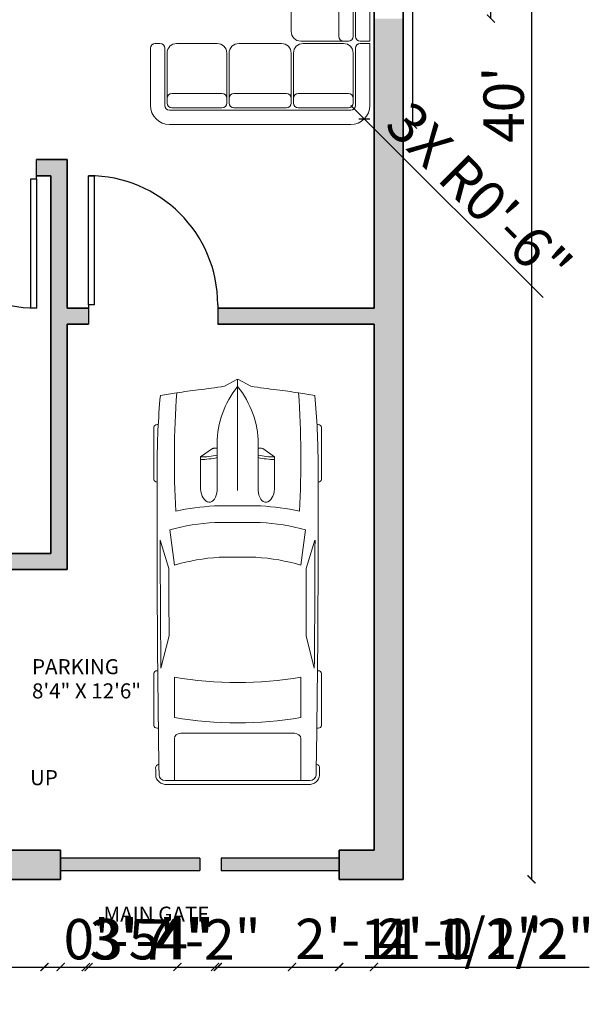
# Model space of a CAD drawing. Units: inches. Extents: x 1750 to 7466, y 1409 to 2004.
# Tile 2 of 5: x 1975 to 2152, y 1409 to 1715. Entities that reach past the tile are written whole.
import ezdxf

# ---------------------------------------------------------------- set-up
doc = ezdxf.new("R2010")
doc.units = ezdxf.units.IN
for name, color, linetype, lineweight in [('A-ANNO-DIMS', 2, 'Continuous', 18), ('A-ANNO-TEXT', 7, 'Continuous', 18), ('A-AREA-IDEN', 7, 'Continuous', 18), ('A-DOOR', 3, 'Continuous', 25), ('A-FURN', 8, 'Continuous', 18), ('A-SITE-PARK', 8, 'Continuous', 13), ('A-WALL', 7, 'Continuous', 35)]:
    doc.layers.add(name, color=color, linetype=linetype, lineweight=lineweight)
doc.layers.add('A-WALL-PATT', color=18, linetype='Continuous', lineweight=13, true_color=0x000000)
doc.styles.get("Standard").update_dxf_attribs({"font": 'arial.ttf'})
doc.dimstyles.new('ISO-25', dxfattribs={"dimtxt": 12.5, "dimasz": 2.5, "dimexe": 1.25, "dimexo": 0.625, "dimtad": 1, "dimdec": 0, "dimlunit": 4, "dimtxsty": 'Standard', "dimblk": 'ARCHTICK', "dimcen": 2.5, "dimse1": 1, "dimse2": 1, "dimclrd": 2, "dimadec": 0, "dimazin": 0, "dimtfac": 1, "dimtdec": 0, "dimtmove": 0, "dimatfit": 3, "dimfxl": 1, "dimarcsym": 0})

# ---------------------------------------------------------------- blocks, each defined once
blk = doc.blocks.new('A$C2AFA021D')
for p, q in [((0.8, 2.3), (0.2, 2.3)), ((0.85, 2.2), (0.85, 2.25)), ((0, 2.1), (0, 0.2)), ((0.15, 0.2), (0.15, 2.1)), ((0.175, 1.55), (0.175, 2.075)), ((0.2, 2.15), (0.8, 2.15)), ((0.225, 2.125), (0.275, 2.125)), ((0.75, 2.125), (0.275, 2.125)), ((0.325, 2.075), (0.325, 1.55)), ((0.85, 1.6), (0.85, 2.025)), ((0.275, 1.5), (0.225, 1.5)), ((0.225, 1.475), (0.275, 1.475)), ((0.275, 1.5), (0.75, 1.5)), ((0.75, 1.475), (0.275, 1.475)), ((0.175, 0.875), (0.175, 1.425)), ((0.325, 1.425), (0.325, 0.875)), ((0.85, 0.925), (0.85, 1.375)), ((0.175, 0.225), (0.175, 0.75)), ((0.275, 0.825), (0.225, 0.825)), ((0.225, 0.8), (0.275, 0.8)), ((0.275, 0.825), (0.75, 0.825)), ((0.75, 0.8), (0.275, 0.8)), ((0.325, 0.75), (0.325, 0.225)), ((0.875, 0.275), (0.875, 0.725)), ((0.975, 0.825), (1.4, 0.825)), ((1.5, 0.725), (1.5, 0.275)), ((1.525, 0.275), (1.525, 0.725)), ((1.625, 0.825), (2.075, 0.825)), ((2.175, 0.725), (2.175, 0.275)), ((2.2, 0.275), (2.2, 0.725)), ((2.3, 0.825), (2.725, 0.825)), ((2.825, 0.725), (2.825, 0.275)), ((2.85, 0.2), (2.85, 0.775)), ((2.9, 0.825), (2.95, 0.825)), ((3, 0.775), (3, 0.2)), ((0.85, 0.275), (0.85, 0.7)), ((1.45, 0.325), (0.925, 0.325)), ((2.125, 0.325), (1.575, 0.325)), ((2.775, 0.325), (2.25, 0.325)), ((0.875, 0.275), (0.875, 0.225)), ((1.5, 0.225), (1.5, 0.275)), ((1.525, 0.275), (1.525, 0.225)), ((2.175, 0.225), (2.175, 0.275)), ((2.2, 0.275), (2.2, 0.225)), ((2.825, 0.225), (2.825, 0.275)), ((0.8, 0.15), (0.2, 0.15)), ((0.275, 0.175), (0.225, 0.175)), ((0.275, 0.175), (0.75, 0.175)), ((0.925, 0.175), (1.45, 0.175)), ((0.925, 0.15), (2.8, 0.15)), ((1.575, 0.175), (2.125, 0.175)), ((2.25, 0.175), (2.775, 0.175)), ((0.85, 0), (0.85, 0.1)), ((0.875, 0.1), (0.875, 0)), ((0.2, 0), (0.85, 0)), ((2.8, 0), (0.875, 0))]:
    blk.add_line(p, q)
for centre, radius, start, end in [((0.2, 2.1), 0.2, 90, 180), ((0.8, 2.25), 0.05, 0, 90), ((0.8, 2.2), 0.05, 270, 0), ((0.2, 2.1), 0.05, 90, 180), ((0.225, 2.075), 0.05, 90, 180), ((0.275, 2.075), 0.05, 0, 90), ((0.75, 2.025), 0.1, 0, 90), ((0.225, 1.55), 0.05, 180, 270), ((0.275, 1.55), 0.05, 270, 0), ((0.75, 1.6), 0.1, 270, 0), ((0.225, 1.425), 0.05, 90, 180), ((0.275, 1.425), 0.05, 0, 90), ((0.75, 1.375), 0.1, 360, 90), ((0.225, 0.875), 0.05, 180, 270), ((0.275, 0.875), 0.05, 270, 0), ((0.75, 0.925), 0.1, 270, 0), ((0.225, 0.75), 0.05, 90, 180), ((0.275, 0.75), 0.05, 0, 90), ((0.75, 0.7), 0.1, 0, 90), ((0.975, 0.725), 0.1, 90, 180), ((1.4, 0.725), 0.1, 0, 90), ((1.625, 0.725), 0.1, 90, 180), ((2.075, 0.725), 0.1, 0, 90), ((2.3, 0.725), 0.1, 90, 180), ((2.725, 0.725), 0.1, 0, 90), ((2.9, 0.775), 0.05, 90, 180), ((2.95, 0.775), 0.05, 0, 90), ((0.925, 0.275), 0.05, 90, 180), ((1.45, 0.275), 0.05, 360, 90), ((1.575, 0.275), 0.05, 90, 180), ((2.125, 0.275), 0.05, 360, 90), ((2.25, 0.275), 0.05, 90, 180), ((2.775, 0.275), 0.05, 360, 90), ((0.225, 0.225), 0.05, 180, 270), ((0.275, 0.225), 0.05, 270, 0), ((0.75, 0.275), 0.1, 270, 0), ((0.925, 0.225), 0.05, 180, 270), ((1.45, 0.225), 0.05, 270, 0), ((1.575, 0.225), 0.05, 180, 270), ((2.125, 0.225), 0.05, 270, 0), ((2.25, 0.225), 0.05, 180, 270), ((2.775, 0.225), 0.05, 270, 0), ((0.2, 0.2), 0.2, 180, 270), ((0.2, 0.2), 0.05, 180, 270), ((0.8, 0.1), 0.05, 0, 90), ((0.925, 0.1), 0.05, 90, 180), ((2.8, 0.2), 0.2, 270, 0), ((2.8, 0.2), 0.05, 270, 0)]:
    blk.add_arc(centre, radius, start, end)
blk = doc.blocks.new('*U12')
for p, q in [((21.1, 37.41), (21.1, 36.83)), ((46.55, 38.89), (22.35, 38.89)), ((47.8, 37.39), (47.8, 37.41)), ((135.45, 37.07), (135.45, 37.41)), ((136.7, 38.89), (160.9, 38.89)), ((162.15, 37.41), (162.15, 36.77)), ((87.99, 31.87), (74.76, 35.92)), ((134.31, 35.6), (119.29, 31.78)), ((186.47, -33.5), (186.47, 33.5)), ((188.4, -32.76), (188.4, 32.76)), ((70.03, 31.54), (86.41, 29.35)), ((138.42, 29.35), (157.25, 29.35)), ((186.47, 29.35), (167.01, 29.35)), ((164.52, 26.39), (164.52, -26.39)), ((32.27, 11.63), (36.13, 17.17)), ((36.13, 17.17), (50.94, 17.17)), ((29.77, 9.51), (51.68, 9.51)), ((32.12, 9.51), (32.12, 11.15)), ((58.92, -10.77), (58.92, 10.77)), ((66.55, -10.53), (66.55, 10.53)), ((186.47, -10.53), (186.47, 10.53)), ((3.27, 6.13), (0.1, 0.41)), ((82.74, 8.5), (82.74, -8.5)), ((0, 0), (51.68, 0)), ((0.1, -0.41), (3.27, -6.13)), ((29.77, -9.51), (51.68, -9.51)), ((32.12, -9.51), (32.12, -11.15)), ((32.27, -11.63), (36.13, -17.17)), ((36.13, -17.17), (50.94, -17.17)), ((86.41, -29.35), (70.03, -31.54)), ((87.99, -31.87), (74.76, -35.92)), ((134.31, -35.6), (119.29, -31.78)), ((157.25, -29.35), (138.42, -29.35)), ((167.01, -29.35), (186.47, -29.35)), ((21.1, -37.41), (21.1, -36.83)), ((46.55, -38.89), (22.35, -38.89)), ((47.8, -37.39), (47.8, -37.41)), ((135.45, -37.07), (135.45, -37.41)), ((136.7, -38.89), (160.9, -38.89)), ((162.15, -37.41), (162.15, -36.77))]:
    blk.add_line(p, q)
for centre, major_axis, ratio, start_param, end_param in [((41.19, -490.86), (0, 528.23), 0.842304, 0.00281, 0.075598), ((22.35, 37.41), (0, -1.48), 0.842304, 3.141593, 4.712389), ((64.48, -10555.62), (0, 10593.03), 0.842304, -0.013397, 0.002797), ((46.55, 37.41), (0, 1.48), 0.842304, -1.570796, 0), ((136.7, 37.41), (0, -1.48), 0.842304, 3.141593, 4.712389), ((160.9, 37.41), (0, 1.48), 0.842304, -1.570796, 0), ((180.63, 35.84), (0, 2.22), 0.842304, -0.013017, 1.249894), ((64.48, -10556.36), (0, 10595.31), 0.842304, -0.013397, -0.013017), ((183.98, 32.76), (0, -5.25), 0.842304, 1.570796, 3.128196), ((266.03, -27.52), (0, 313.31), 0.842304, 1.367076, 1.39176), ((64.48, -10555.62), (0, -10591.55), 0.842304, 3.133765, 3.140441), ((183.98, 33.5), (0, -2.96), 0.842304, 1.570796, 3.128196), ((259.18, -27.52), (0, -305.3), 0.842304, 4.528606, 4.561838), ((37.47, -593.96), (0, -623.33), 0.842304, 3.096046, 3.200911), ((134.4, 5.39), (0, -89.78), 0.842304, 4.449482, 4.652344), ((135.29, 5.39), (0, 81.77), 0.842304, 1.245306, 1.50788), ((149.6, 2.8), (0, -79.58), 0.842304, 4.372215, 4.640744), ((95.79, -3666.35), (0, -3698.24), 0.842304, 3.134049, 3.144098), ((17.08, 0), (0, 147.02), 0.842304, 4.511394, 4.913384), ((35.91, 0), (0, 147.02), 0.842304, 4.511394, 4.913384), ((167.01, 26.39), (0, 2.96), 0.842304, 0, 1.570796), ((-204.49, 52.4), (0, -250.96), 0.842304, 1.385369, 1.434372), ((13.04, 17.01), (0, 27.42), 0.842304, 4.435146, 4.718221), ((14.2, 17.01), (0, 27.42), 0.842304, 4.435146, 4.718221), ((50.79, 13.34), (6.34, -0.36), 0.603834, -1.395552, 1.581315), ((29.77, -46.66), (0, 56.17), 0.842304, 0, 0.590319), ((32.75, 11.15), (0, 0.74), 0.842304, 0.879714, 1.570796), ((0.62, 0), (0, -0.74), 0.842304, 4.131459, 5.293319), ((29.77, 46.66), (0, 56.17), 0.842304, 2.551274, 3.141593), ((-204.49, -52.4), (0, 250.96), 0.842304, -1.434372, -1.385369), ((149.6, -2.8), (0, -79.58), 0.842304, -1.499151, -1.230623), ((32.75, -11.15), (0, -0.74), 0.842304, 4.712389, 5.403472), ((13.04, -17.01), (0, -27.42), 0.842304, 1.564964, 1.848039), ((14.2, -17.01), (0, -27.42), 0.842304, 1.564964, 1.848039), ((134.4, -5.39), (0, -89.78), 0.842304, -1.510751, -1.307889), ((135.29, -5.39), (0, -81.77), 0.842304, -1.50788, -1.245306), ((259.18, 27.52), (0, 305.3), 0.842304, 1.721348, 1.754579), ((167.01, -26.39), (0, -2.96), 0.842304, 4.712389, 6.283185), ((266.03, 27.52), (0, 313.31), 0.842304, 1.749832, 1.774517), ((37.47, 593.96), (0, -623.33), 0.842304, -0.059319, 0.045547), ((95.79, 3666.35), (0, -3698.24), 0.842304, -0.002505, 0.007544), ((41.19, 490.86), (0, -528.23), 0.842304, -0.075598, -0.00281), ((64.48, 10555.62), (0, 10593.03), 0.842304, 3.138796, 3.15499), ((64.48, 10555.62), (0, -10591.55), 0.842304, 0.001152, 0.007828), ((180.63, -35.84), (0, -2.22), 0.842304, -1.249894, 0.013017), ((183.98, -33.5), (0, 2.96), 0.842304, 3.15499, 4.712389), ((183.98, -32.76), (0, -5.25), 0.842304, 0.013397, 1.570796), ((22.35, -37.41), (0, 1.48), 0.842304, 1.570796, 3.141593), ((46.55, -37.41), (0, -1.48), 0.842304, 0, 1.570796), ((136.7, -37.41), (0, -1.48), 0.842304, -1.570796, 0), ((160.9, -37.41), (0, 1.48), 0.842304, 3.141593, 4.712389), ((64.48, 10556.36), (0, 10595.31), 0.842304, 3.15461, 3.15499)]:
    blk.add_ellipse(centre, major_axis=major_axis, ratio=ratio, start_param=start_param, end_param=end_param)
at = {"extrusion": (0, 0, -1)}
blk.add_ellipse((50.79, -13.34), major_axis=(6.34, 0.36), ratio=0.603834, start_param=-1.395552, end_param=1.581315, dxfattribs=at)
blk = doc.blocks.new('*U11')
for p, q in [((0, 0), (0, -6)), ((40, 0), (40, -6))]:
    blk.add_line(p, q)
blk.add_lwpolyline([(0, 0), (0, 40), (1.75, 40), (1.75, 0)], close=True)
blk.add_arc((0, 0), 40, 0, 90)
blk = doc.blocks.new('_ArchTick')
at = {"color": 0, "linetype": 'ByBlock', "const_width": 0.15}
blk.add_lwpolyline([(-0.5, -0.5), (0.5, 0.5)], dxfattribs=at)
blk = doc.blocks.new('*D14')
at = {"layer": 'A-ANNO-DIMS', "color": 0, "lineweight": -2, "transparency": 16777216}
blk.add_line((2133.87, 1928.17), (2133.87, 1448.17), dxfattribs=at)
at = {"layer": 'Defpoints', "color": 0, "transparency": 16777216}
for p in [(2094.13, 1928.17), (2094.13, 1448.17), (2133.87, 1448.17)]:
    blk.add_point(p, dxfattribs=at)
at = {"layer": 'A-ANNO-DIMS', "color": 0, "lineweight": -2, "transparency": 16777216, "xscale": 2.5, "yscale": 2.5, "zscale": 2.5}
for p, rotation in [((2133.87, 1928.17), 90), ((2133.87, 1448.17), 270)]:
    blk.add_blockref('_ArchTick', p, dxfattribs=dict(at, rotation=rotation))
at = {"layer": 'A-ANNO-DIMS', "color": 0, "transparency": 16777216, "insert": (2126.86, 1688.17), "char_height": 12.5, "attachment_point": 5, "rotation": 90}
blk.add_mtext("40'", dxfattribs=at)
blk = doc.blocks.new('*D17')
at = {"layer": 'A-ANNO-DIMS', "color": 2, "lineweight": -2, "transparency": 16777216}
for p, q in [((2097.12, 1770.61), (2097.12, 1889.05)), ((2097.12, 1682.03), (2097.12, 1770.61))]:
    blk.add_line(p, q, dxfattribs=at)
at = {"layer": 'Defpoints', "color": 0, "transparency": 16777216}
for p in [(2083.83, 1770.61), (2097.12, 1770.61), (2083.83, 1682.03)]:
    blk.add_point(p, dxfattribs=at)
at = {"layer": 'A-ANNO-DIMS', "color": 2, "lineweight": -2, "transparency": 16777216, "xscale": 2.5, "yscale": 2.5, "zscale": 2.5}
for p, rotation in [((2097.12, 1770.61), 90), ((2097.12, 1682.03), 270)]:
    blk.add_blockref('_ArchTick', p, dxfattribs=dict(at, rotation=rotation))
at = {"layer": 'A-ANNO-DIMS', "color": 0, "transparency": 16777216, "insert": (2090.03, 1831.08), "char_height": 12.5, "attachment_point": 5, "rotation": 90}
blk.add_mtext('SOFA 7\'-4 1/2"', dxfattribs=at)
blk = doc.blocks.new('*D25')
at = {"layer": 'A-ANNO-DIMS', "color": 2, "lineweight": -2, "transparency": 16777216}
blk.add_line((1988.13, 1421.02), (2074.33, 1421.02), dxfattribs=at)
at = {"layer": 'Defpoints', "color": 0, "transparency": 16777216}
for p in [(1988.13, 1448.17), (2074.33, 1448.17), (2074.33, 1421.02)]:
    blk.add_point(p, dxfattribs=at)
at = {"layer": 'A-ANNO-DIMS', "color": 2, "lineweight": -2, "transparency": 16777216, "xscale": 2.5, "yscale": 2.5, "zscale": 2.5, "rotation": 180}
blk.add_blockref('_ArchTick', (1988.13, 1421.02), dxfattribs=at)
at = {"layer": 'A-ANNO-DIMS', "color": 2, "lineweight": -2, "transparency": 16777216, "xscale": 2.5, "yscale": 2.5, "zscale": 2.5}
blk.add_blockref('_ArchTick', (2074.33, 1421.02), dxfattribs=at)
at = {"layer": 'A-ANNO-DIMS', "color": 0, "transparency": 16777216, "insert": (2031.23, 1427.92), "char_height": 12.5, "attachment_point": 5}
blk.add_mtext('7\'-2"', dxfattribs=at)
blk = doc.blocks.new('*D26')
at = {"layer": 'A-ANNO-DIMS', "color": 2, "lineweight": -2, "transparency": 16777216}
blk.add_line((1854.13, 1421.02), (1988.13, 1421.02), dxfattribs=at)
at = {"layer": 'Defpoints', "color": 0, "transparency": 16777216}
for p in [(1854.13, 1448.17), (1988.13, 1448.17), (1988.13, 1421.02)]:
    blk.add_point(p, dxfattribs=at)
at = {"layer": 'A-ANNO-DIMS', "color": 2, "lineweight": -2, "transparency": 16777216, "xscale": 2.5, "yscale": 2.5, "zscale": 2.5, "rotation": 180}
blk.add_blockref('_ArchTick', (1854.13, 1421.02), dxfattribs=at)
at = {"layer": 'A-ANNO-DIMS', "color": 2, "lineweight": -2, "transparency": 16777216, "xscale": 2.5, "yscale": 2.5, "zscale": 2.5}
blk.add_blockref('_ArchTick', (1988.13, 1421.02), dxfattribs=at)
at = {"layer": 'A-ANNO-DIMS', "color": 0, "transparency": 16777216, "insert": (1921.13, 1427.92), "char_height": 12.5, "attachment_point": 5}
blk.add_mtext('11\'-2"', dxfattribs=at)
blk = doc.blocks.new('*D38')
at = {"layer": 'A-ANNO-DIMS', "color": 2, "lineweight": -2, "transparency": 16777216}
for p, q in [((2024.28, 1421.02), (2059.72, 1421.02)), ((2059.72, 1421.02), (2135.75, 1421.02))]:
    blk.add_line(p, q, dxfattribs=at)
at = {"layer": 'Defpoints', "color": 0, "transparency": 16777216}
for p in [(2024.28, 1889.13), (2059.72, 1889.13), (2059.72, 1421.02)]:
    blk.add_point(p, dxfattribs=at)
at = {"layer": 'A-ANNO-DIMS', "color": 2, "lineweight": -2, "transparency": 16777216, "xscale": 2.5, "yscale": 2.5, "zscale": 2.5, "rotation": 180}
blk.add_blockref('_ArchTick', (2024.28, 1421.02), dxfattribs=at)
at = {"layer": 'A-ANNO-DIMS', "color": 2, "lineweight": -2, "transparency": 16777216, "xscale": 2.5, "yscale": 2.5, "zscale": 2.5}
blk.add_blockref('_ArchTick', (2059.72, 1421.02), dxfattribs=at)
at = {"layer": 'A-ANNO-DIMS', "color": 0, "transparency": 16777216, "insert": (2098.98, 1428.1), "char_height": 12.5, "attachment_point": 5}
blk.add_mtext('2\'-11 1/2"', dxfattribs=at)
blk = doc.blocks.new('*D40')
at = {"layer": 'A-ANNO-DIMS', "color": 2, "lineweight": -2, "transparency": 16777216}
for p, q in [((2059.72, 1421.02), (2085.13, 1421.02)), ((2085.13, 1421.02), (2151.45, 1421.02))]:
    blk.add_line(p, q, dxfattribs=at)
at = {"layer": 'Defpoints', "color": 0, "transparency": 16777216}
for p in [(2059.72, 1804.17), (2085.13, 1804.17), (2085.13, 1421.02)]:
    blk.add_point(p, dxfattribs=at)
at = {"layer": 'A-ANNO-DIMS', "color": 2, "lineweight": -2, "transparency": 16777216, "xscale": 2.5, "yscale": 2.5, "zscale": 2.5, "rotation": 180}
blk.add_blockref('_ArchTick', (2059.72, 1421.02), dxfattribs=at)
at = {"layer": 'A-ANNO-DIMS', "color": 2, "lineweight": -2, "transparency": 16777216, "xscale": 2.5, "yscale": 2.5, "zscale": 2.5}
blk.add_blockref('_ArchTick', (2085.13, 1421.02), dxfattribs=at)
at = {"layer": 'A-ANNO-DIMS', "color": 0, "transparency": 16777216, "insert": (2119.54, 1428.1), "char_height": 12.5, "attachment_point": 5}
blk.add_mtext('2\'-1 1/2"', dxfattribs=at)
blk = doc.blocks.new('*D41')
at = {"layer": 'A-ANNO-DIMS', "color": 2, "lineweight": -2, "transparency": 16777216}
blk.add_line((1995.93, 1421.02), (2035.93, 1421.02), dxfattribs=at)
at = {"layer": 'Defpoints', "color": 0, "transparency": 16777216}
for p in [(1995.93, 1804.17), (2035.93, 1804.17), (2035.93, 1421.02)]:
    blk.add_point(p, dxfattribs=at)
at = {"layer": 'A-ANNO-DIMS', "color": 2, "lineweight": -2, "transparency": 16777216, "xscale": 2.5, "yscale": 2.5, "zscale": 2.5, "rotation": 180}
blk.add_blockref('_ArchTick', (1995.93, 1421.02), dxfattribs=at)
at = {"layer": 'A-ANNO-DIMS', "color": 2, "lineweight": -2, "transparency": 16777216, "xscale": 2.5, "yscale": 2.5, "zscale": 2.5}
blk.add_blockref('_ArchTick', (2035.93, 1421.02), dxfattribs=at)
at = {"layer": 'A-ANNO-DIMS', "color": 0, "transparency": 16777216, "insert": (2015.93, 1428.03), "char_height": 12.5, "attachment_point": 5}
blk.add_mtext('3\'-4"', dxfattribs=at)
blk = doc.blocks.new('*D48')
at = {"layer": 'A-ANNO-DIMS', "color": 2, "lineweight": -2, "transparency": 16777216}
for p, q in [((1983.13, 1421.02), (1988.13, 1421.02)), ((1988.13, 1421.02), (2025.11, 1421.02))]:
    blk.add_line(p, q, dxfattribs=at)
at = {"layer": 'Defpoints', "color": 0, "transparency": 16777216}
for p in [(1983.13, 1804.17), (1988.13, 1804.17), (1988.13, 1421.02)]:
    blk.add_point(p, dxfattribs=at)
at = {"layer": 'A-ANNO-DIMS', "color": 2, "lineweight": -2, "transparency": 16777216, "xscale": 2.5, "yscale": 2.5, "zscale": 2.5, "rotation": 180}
blk.add_blockref('_ArchTick', (1983.13, 1421.02), dxfattribs=at)
at = {"layer": 'A-ANNO-DIMS', "color": 2, "lineweight": -2, "transparency": 16777216, "xscale": 2.5, "yscale": 2.5, "zscale": 2.5}
blk.add_blockref('_ArchTick', (1988.13, 1421.02), dxfattribs=at)
at = {"layer": 'A-ANNO-DIMS', "color": 0, "transparency": 16777216, "insert": (2007.87, 1428.02), "char_height": 12.5, "attachment_point": 5}
blk.add_mtext('0\'-5"', dxfattribs=at)
blk = doc.blocks.new('*D51')
at = {"layer": 'A-ANNO-DIMS', "color": 2, "lineweight": -2, "transparency": 16777216}
blk.add_line((1996.77, 1421.02), (2036.77, 1421.02), dxfattribs=at)
at = {"layer": 'Defpoints', "color": 0, "transparency": 16777216}
for p in [(1996.77, 1620.17), (2036.77, 1620.17), (2036.77, 1421.02)]:
    blk.add_point(p, dxfattribs=at)
at = {"layer": 'A-ANNO-DIMS', "color": 2, "lineweight": -2, "transparency": 16777216, "xscale": 2.5, "yscale": 2.5, "zscale": 2.5, "rotation": 180}
blk.add_blockref('_ArchTick', (1996.77, 1421.02), dxfattribs=at)
at = {"layer": 'A-ANNO-DIMS', "color": 2, "lineweight": -2, "transparency": 16777216, "xscale": 2.5, "yscale": 2.5, "zscale": 2.5}
blk.add_blockref('_ArchTick', (2036.77, 1421.02), dxfattribs=at)
at = {"layer": 'A-ANNO-DIMS', "color": 0, "transparency": 16777216, "insert": (2016.77, 1428.03), "char_height": 12.5, "attachment_point": 5}
blk.add_mtext('3\'-4"', dxfattribs=at)
blk = doc.blocks.new('*D52')
at = {"layer": 'A-ANNO-DIMS', "color": 2, "lineweight": -2, "transparency": 16777216}
for p, q in [((2036.77, 1421.02), (2085.13, 1421.02)), ((2085.13, 1421.02), (2151.74, 1421.02))]:
    blk.add_line(p, q, dxfattribs=at)
at = {"layer": 'Defpoints', "color": 0, "transparency": 16777216}
for p in [(2036.77, 1620.17), (2085.13, 1620.17), (2085.13, 1421.02)]:
    blk.add_point(p, dxfattribs=at)
at = {"layer": 'A-ANNO-DIMS', "color": 2, "lineweight": -2, "transparency": 16777216, "xscale": 2.5, "yscale": 2.5, "zscale": 2.5, "rotation": 180}
blk.add_blockref('_ArchTick', (2036.77, 1421.02), dxfattribs=at)
at = {"layer": 'A-ANNO-DIMS', "color": 2, "lineweight": -2, "transparency": 16777216, "xscale": 2.5, "yscale": 2.5, "zscale": 2.5}
blk.add_blockref('_ArchTick', (2085.13, 1421.02), dxfattribs=at)
at = {"layer": 'A-ANNO-DIMS', "color": 0, "transparency": 16777216, "insert": (2119.69, 1428.1), "char_height": 12.5, "attachment_point": 5}
blk.add_mtext('4\'-0 1/2"', dxfattribs=at)
blk = doc.blocks.new('*D53')
at = {"layer": 'A-ANNO-DIMS', "color": 2, "lineweight": -2, "transparency": 16777216}
for p, q in [((2121.28, 1763.18), (2121.28, 1829.79)), ((2121.28, 1714.84), (2121.28, 1763.18))]:
    blk.add_line(p, q, dxfattribs=at)
at = {"layer": 'Defpoints', "color": 0, "transparency": 16777216}
for p in [(2094.13, 1763.18), (2121.28, 1763.18), (2094.13, 1714.84)]:
    blk.add_point(p, dxfattribs=at)
at = {"layer": 'A-ANNO-DIMS', "color": 2, "lineweight": -2, "transparency": 16777216, "xscale": 2.5, "yscale": 2.5, "zscale": 2.5}
for p, rotation in [((2121.28, 1763.18), 90), ((2121.28, 1714.84), 270)]:
    blk.add_blockref('_ArchTick', p, dxfattribs=dict(at, rotation=rotation))
at = {"layer": 'A-ANNO-DIMS', "color": 0, "transparency": 16777216, "insert": (2114.2, 1797.73), "char_height": 12.5, "attachment_point": 5, "rotation": 90}
blk.add_mtext('4\'-0 1/2"', dxfattribs=at)
blk = doc.blocks.new('*D56')
at = {"layer": 'A-ANNO-DIMS', "color": 2, "lineweight": -2, "transparency": 16777216}
for p in [(2077.93, 1687.93), (2137.46, 1628.4)]:
    blk.add_line(p, (2082.1, 1683.76), dxfattribs=at)
at = {"layer": 'Defpoints', "color": 0, "transparency": 16777216}
for p in [(2077.93, 1687.93), (2082.1, 1683.76)]:
    blk.add_point(p, dxfattribs=at)
at = {"layer": 'A-ANNO-DIMS', "color": 2, "lineweight": -2, "transparency": 16777216, "xscale": 2.5, "yscale": 2.5, "zscale": 2.5, "rotation": 135.0003567295032}
blk.add_blockref('_ArchTick', (2082.1, 1683.76), dxfattribs=at)
at = {"layer": 'A-ANNO-DIMS', "color": 0, "transparency": 16777216, "insert": (2116.51, 1659.27), "char_height": 12.5, "attachment_point": 5, "rotation": 315.0004}
blk.add_mtext('3X R0\'-6"', dxfattribs=at)

msp = doc.modelspace()

# ---------------------------------------------------------------- hatches: boundary and pattern name
at = {"layer": 'A-WALL-PATT'}
h = msp.add_hatch(color=256, dxfattribs=at)
h.dxf.hatch_style = 1
h.paths.add_polyline_path([(1896.49, 1928.17), (1854.13, 1928.17), (1854.13, 1893.52), (1863.13, 1893.52), (1863.13, 1919.17), (1896.49, 1919.17)])
h.paths.add_polyline_path([(2022.32, 1928.17), (1945.82, 1928.17), (1945.82, 1919.17), (1983.13, 1919.17), (1983.13, 1804.17), (1974.13, 1804.17), (1974.13, 1799.17), (1995.93, 1799.17), (1995.93, 1804.17), (1988.13, 1804.17), (1988.13, 1919.17), (2022.32, 1919.17)])
h.paths.add_polyline_path([(2094.13, 1928.17), (2070.34, 1928.17), (2070.34, 1919.17), (2085.13, 1919.17), (2085.13, 1875.24), (2094.13, 1875.24)])
h.paths.add_polyline_path([(2094.13, 1827.64), (2085.13, 1827.64), (2085.13, 1804.17), (2035.93, 1804.17), (2035.93, 1799.17), (2085.13, 1799.17), (2085.13, 1763.18), (2094.13, 1763.18)])
h.paths.add_polyline_path([(1863.13, 1846.52), (1854.13, 1846.52), (1854.13, 1751.88), (1863.13, 1751.88)])
h.paths.add_polyline_path([(1934.13, 1804.17), (1863.13, 1804.17), (1863.13, 1799.17), (1911.13, 1799.17), (1911.13, 1794.68), (1912.55, 1794.68), (1916.13, 1794.68), (1916.13, 1799.17), (1934.13, 1799.17)])
h.paths.add_polyline_path([(1863.13, 1726.23), (1854.13, 1726.23), (1854.13, 1709.82), (1863.13, 1709.82), (1863.13, 1714.17), (1911.13, 1714.17), (1911.13, 1671.17), (1887.9, 1671.17, -0.01479), (1887.95, 1669.75), (1887.95, 1666.17), (1916.13, 1666.17), (1940.64, 1666.17), (1940.64, 1671.17), (1916.13, 1671.17), (1916.13, 1770.77), (1912.55, 1770.77, -0.01479), (1911.13, 1770.81), (1911.13, 1719.17), (1863.13, 1719.17)])
h.paths.add_polyline_path([(1863.13, 1684.17), (1854.13, 1684.17), (1854.13, 1625.24), (1863.13, 1625.24)])
h.paths.add_polyline_path([(1863.13, 1577.33), (1854.13, 1577.33), (1854.13, 1526.31), (1863.13, 1526.31), (1863.13, 1544.17), (1983.13, 1544.17), (1988.13, 1544.17), (1990.13, 1544.17), (1990.13, 1549.17), (1990.13, 1620.17), (1996.77, 1620.17), (1996.77, 1625.17), (1990.13, 1625.17), (1990.13, 1666.17), (1990.13, 1671.17), (1980.64, 1671.17), (1980.64, 1666.17), (1985.13, 1666.17), (1985.13, 1625.17), (1985.13, 1549.17), (1863.13, 1549.17)])
h.paths.add_polyline_path([(1988.13, 1457.17), (1863.13, 1457.17), (1863.13, 1497.36), (1854.13, 1497.36), (1854.13, 1448.17), (1988.13, 1448.17)])
h.paths.add_polyline_path([(2031.23, 1454.78), (1988.13, 1454.78), (1988.13, 1450.91), (2031.23, 1450.91)])
h.paths.add_polyline_path([(2074.33, 1454.78), (2037.79, 1454.78), (2037.79, 1450.91), (2074.33, 1450.91)], flags=17)
h.paths.add_polyline_path([(2094.13, 1714.84), (2085.13, 1714.84), (2085.13, 1625.17), (2036.77, 1625.17), (2036.77, 1620.17), (2085.13, 1620.17), (2085.13, 1457.17), (2074.33, 1457.17), (2074.33, 1448.17), (2094.13, 1448.17)])
h.paths.add_polyline_path([(1846.92, 1867), (1855.4, 1867), (1855.4, 1874), (1846.92, 1874)], flags=9)
h.paths.add_polyline_path([(1885.75, 1686.15), (1909.97, 1686.15), (1909.97, 1693.31), (1885.75, 1693.31)], flags=25)
h.paths.add_polyline_path([(1885.73, 1693.64), (1900.82, 1693.64), (1900.82, 1700.88), (1885.73, 1700.88)], flags=25)
h.paths.add_polyline_path([(1866.42, 1762.99), (1892.45, 1762.99), (1892.45, 1770.14), (1866.42, 1770.14)], flags=25)
h.paths.add_polyline_path([(1866.4, 1770.47), (1898.87, 1770.47), (1898.87, 1777.71), (1866.4, 1777.71)], flags=9)
h.paths.add_polyline_path([(1925.02, 1731.07), (1964.24, 1731.07), (1964.24, 1738.22), (1925.02, 1738.22)], flags=9)
h.paths.add_polyline_path([(1925.01, 1738.55), (1982.11, 1738.55), (1982.11, 1745.79), (1925.01, 1745.79)], flags=9)
h.paths.add_polyline_path([(1995.48, 1862.99), (2034.71, 1862.99), (2034.71, 1870.14), (1995.48, 1870.14)], flags=9)
h.paths.add_polyline_path([(1995.47, 1870.47), (2026.49, 1870.47), (2026.49, 1877.71), (1995.47, 1877.71)], flags=9)
h.paths.add_polyline_path([(1869.07, 1829.02), (1905.98, 1829.02), (1905.98, 1836.17), (1869.07, 1836.17)], flags=9)
h.paths.add_polyline_path([(1869.05, 1836.5), (1905.15, 1836.5), (1905.15, 1843.74), (1869.05, 1843.74)], flags=9)

# ---------------------------------------------------------------- linework, layer by layer
at = {"layer": 'A-DOOR'}
for p, q in [((1988.13, 1454.78), (1988.13, 1450.91)), ((2031.23, 1454.78), (1988.13, 1454.78)), ((2031.23, 1454.78), (2031.23, 1450.91)), ((2074.33, 1454.78), (2037.79, 1454.78)), ((2037.79, 1454.78), (2037.79, 1450.91)), ((1988.13, 1450.91), (2031.23, 1450.91)), ((2037.79, 1450.91), (2074.33, 1450.91))]:
    msp.add_line(p, q, dxfattribs=at)
at = {"layer": 'A-WALL'}
for p, q in [((2085.13, 1799.17), (2085.13, 1625.17)), ((1990.13, 1671.17), (1980.64, 1671.17)), ((1990.13, 1666.17), (1990.13, 1671.17)), ((1985.13, 1666.17), (1980.64, 1666.17)), ((1985.13, 1625.17), (1985.13, 1666.17)), ((1990.13, 1625.17), (1990.13, 1666.17)), ((1985.13, 1549.17), (1985.13, 1625.17)), ((1990.13, 1625.17), (1996.77, 1625.17)), ((2036.77, 1625.17), (2085.13, 1625.17)), ((1990.13, 1549.17), (1990.13, 1620.17)), ((1990.13, 1620.17), (1996.77, 1620.17)), ((2036.77, 1620.17), (2085.13, 1620.17)), ((2085.13, 1620.17), (2085.13, 1457.17)), ((1863.13, 1549.17), (1985.13, 1549.17)), ((1990.13, 1549.17), (1990.13, 1544.17)), ((1863.13, 1544.17), (1983.13, 1544.17)), ((1983.13, 1544.17), (1988.13, 1544.17)), ((1988.13, 1544.17), (1990.13, 1544.17)), ((1988.13, 1457.17), (1863.13, 1457.17)), ((1988.13, 1457.17), (1988.13, 1448.17)), ((2085.13, 1457.17), (2074.33, 1457.17)), ((2074.33, 1457.17), (2074.33, 1448.17))]:
    msp.add_line(p, q, dxfattribs=at)
msp.add_lwpolyline([(1988.13, 1448.17), (1854.13, 1448.17), (1854.13, 1928.17), (2094.13, 1928.17), (2094.13, 1448.17), (2074.33, 1448.17)], dxfattribs=at)

# ---------------------------------------------------------------- block references
at = {"layer": 'A-DOOR', "rotation": 180}
msp.add_blockref('*U11', (1980.64, 1665.17), dxfattribs=at)
at = {"layer": 'A-DOOR'}
msp.add_blockref('*U11', (1996.77, 1626.17), dxfattribs=at)
at = {"layer": 'A-FURN', "xscale": 29.52853756539839, "yscale": 29.52853756539839, "zscale": 29.52853756539839, "rotation": 90}
msp.add_blockref('A$C2AFA021D', (2083.83, 1682.03), dxfattribs=at)
at = {"layer": 'A-SITE-PARK', "xscale": 0.6667496230024346, "yscale": 0.6667496230024346, "zscale": 0.6667496230024346, "rotation": 270}
msp.add_blockref('*U12', (2042.9, 1603.13), dxfattribs=at)

# ---------------------------------------------------------------- texts
at = {"layer": 'A-ANNO-TEXT'}
for s, p in [('UP', (1978.64, 1477.35)), ('MAIN GATE', (2001.39, 1435.06))]:
    msp.add_text(s, height=4.666, dxfattribs=at).set_placement(p)
at = {"layer": 'A-AREA-IDEN'}
for s, height, p in [('PARKING', 4.666, (1979.27, 1511.73)), ('8\'4" X 12\'6"', 4.6662, (1979.27, 1504.23))]:
    msp.add_text(s, height=height, dxfattribs=at).set_placement(p)

# ---------------------------------------------------------------- dimensions: what is measured, and where the dimension line sits
at = {"layer": 'A-ANNO-DIMS'}
for base, p1, p2, override, picture, middle in [((2133.87, 1448.17), (2094.13, 1928.17), (2094.13, 1448.17), {"dimclrd": 0, "dimclre": 0, "dimclrt": 0}, '*D14', (2126.86, 1688.17)), ((2121.28, 1763.18), (2094.13, 1714.84), (2094.13, 1763.18), {"dimdec": 1, "dimlfac": 1, "dimrnd": 0, "dimzin": 1, "dimdsep": 46, "dimlunit": 4, "dimfrac": 2}, '*D53', (2114.2, 1797.73))]:
    dim = msp.add_linear_dim(base=base, p1=p1, p2=p2, angle=90, dimstyle='ISO-25', override=override, dxfattribs=at)
    dim.commit()
    dim.dimension.update_dxf_attribs({"geometry": picture, "text_midpoint": middle})
for base, p1, p2, picture, middle in [((2059.72, 1421.02), (2024.28, 1889.13), (2059.72, 1889.13), '*D38', (2098.98, 1428.1)), ((1988.13, 1421.02), (1983.13, 1804.17), (1988.13, 1804.17), '*D48', (2007.87, 1428.02)), ((2035.93, 1421.02), (1995.93, 1804.17), (2035.93, 1804.17), '*D41', (2015.93, 1428.03)), ((2085.13, 1421.02), (2059.72, 1804.17), (2085.13, 1804.17), '*D40', (2119.54, 1428.1)), ((2036.77, 1421.02), (1996.77, 1620.17), (2036.77, 1620.17), '*D51', (2016.77, 1428.03)), ((2085.13, 1421.02), (2036.77, 1620.17), (2085.13, 1620.17), '*D52', (2119.69, 1428.1)), ((1988.13, 1421.02), (1854.13, 1448.17), (1988.13, 1448.17), '*D26', (1921.13, 1427.92)), ((2074.33, 1421.02), (1988.13, 1448.17), (2074.33, 1448.17), '*D25', (2031.23, 1427.92))]:
    dim = msp.add_linear_dim(base=base, p1=p1, p2=p2, dimstyle='ISO-25', override={"dimdec": 1, "dimlfac": 1, "dimrnd": 0, "dimzin": 1, "dimdsep": 46, "dimlunit": 4, "dimfrac": 2}, dxfattribs=at)
    dim.commit()
    dim.dimension.update_dxf_attribs({"geometry": picture, "text_midpoint": middle})
dim = msp.add_linear_dim(base=(2097.12, 1770.61), p1=(2083.83, 1682.03), p2=(2083.83, 1770.61), angle=90, text='SOFA <>', dimstyle='ISO-25', override={"dimdec": 1, "dimlfac": 1, "dimrnd": 0, "dimzin": 1, "dimdsep": 46, "dimlunit": 4, "dimfrac": 2}, dxfattribs=at)
dim.commit()
dim.dimension.update_dxf_attribs({"geometry": '*D17', "text_midpoint": (2090.03, 1831.08)})
dim = msp.add_radius_dim(center=(2077.93, 1687.93), mpoint=(2082.1, 1683.76), text='3X <>', dimstyle='ISO-25', override={"dimdec": 1, "dimlfac": 1, "dimrnd": 0, "dimzin": 1, "dimdsep": 46, "dimlunit": 4, "dimfrac": 2}, dxfattribs=at)
dim.commit()
dim.dimension.update_dxf_attribs({"geometry": '*D56', "text_midpoint": (2116.51, 1659.27)})

doc.saveas('drawing.dxf')
